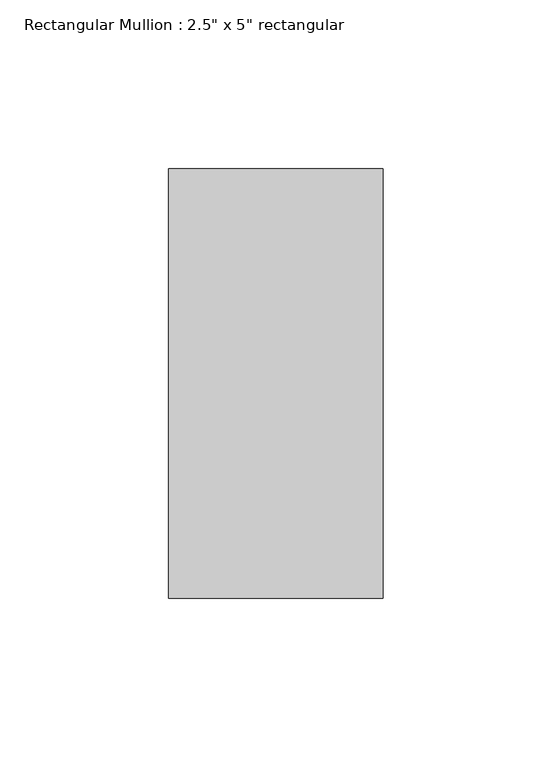
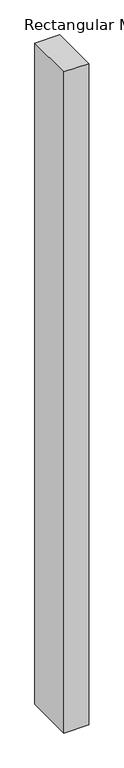
"""IFC4 building model written with IfcOpenShell, lengths in millimetres: member geometry."""

from ifc_helpers import new_model, si_unit, frame, origin, place, context, project, spatial, polyline, outline, extrude, source, transform, mapped, element, save


def member_6e7b816b(model_context):
    return source(origin(), model_context, "Body", "SweptSolid", [
        extrude(outline(polyline([(0.0, 63.5), (0.0, -63.5), (-63.5, -63.5), (-63.5, 63.5), (0.0, 63.5)])), frame((0.0, 0.0, -1770.7328538), z_axis=(0.0, 0.0, 1.0), x_axis=(1.0, 0.0, 0.0)), (0.0, 0.0, 1.0), 1770.7328538),
    ])


if __name__ == "__main__":
    model = new_model("IFC4")
    model_context = context("Model", 3, world=origin())
    ifc_project = project(units=[si_unit("LENGTHUNIT", "METRE", prefix="MILLI")], contexts=[model_context])
    site = spatial("IfcSite", under=ifc_project)
    building = spatial("IfcBuilding", under=site)
    placement = place(None, origin())
    member_shape = member_6e7b816b(model_context)
    element("IfcMember", 1, ObjectType="Rectangular Mullion : 2.5\" x 5\" rectangular", at=placement, inside=building, context=model_context, shape_type="MappedRepresentation", body=[
        mapped(member_shape, transform((0.0, 0.0, 0.0), x_axis=(1.0, 0.0, 0.0), y_axis=(0.0, 1.0, 0.0), z_axis=(0.0, 0.0, 1.0))),
    ])
    save(model, "model.ifc")

# Revit data of these elements
# Type "Rectangular Mullion : 2.5\" x 5\" rectangular"
#   built-in parameter 1007304 = 0.416667 (stored number, unit not read)
#   built-in parameter 1007301 = 0.104167 (stored number, unit not read)
#   built-in parameter 1007300 = 0.104167 (stored number, unit not read)
# Element 1 (IfcMember, "Rectangular Mullion : 2.5\" x 5\" rectangular")
#   Materials on its faces: "Aluminum"
# Materials
#   "Aluminum": class "Metal", colour RGB 247 247 247, transparency 0, Description = "Aluminum 6061", Cost = 0
